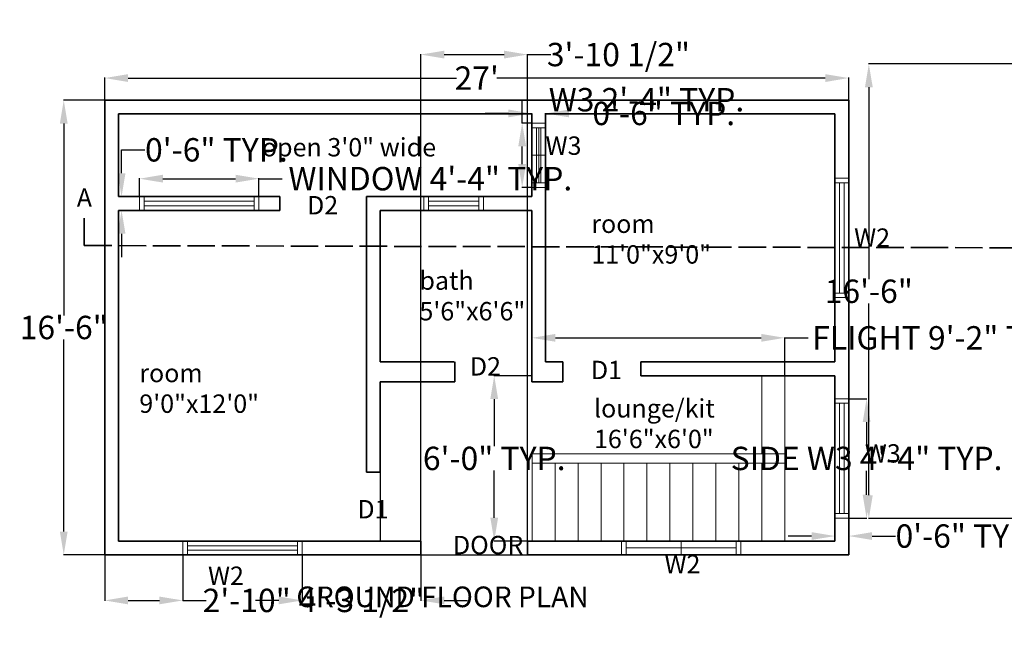
# Model space of a CAD drawing. Units: inches. Extents: x 2393 to 3270, y 740 to 1442.
# Tile 1 of 5: x 2394 to 2823, y 740 to 1008. Entities that reach past the tile are written whole.
import ezdxf

# ---------------------------------------------------------------- set-up
doc = ezdxf.new("R2010")
doc.units = ezdxf.units.IN
doc.header["$MEASUREMENT"] = 0
doc.linetypes.add('ACAD_ISO02W100', pattern=[15, 12, -3])
for name, color, linetype, lineweight in [('A-ANNO-DIMS', 2, 'Continuous', 18), ('A-ANNO-SECT', 1, 'ACAD_ISO02W100', 35), ('A-ANNO-SYMB', 3, 'Continuous', 18), ('A-ANNO-TEXT', 7, 'Continuous', 18), ('A-ANNO-TITL', 7, 'Continuous', 25), ('A-AREA-IDEN', 7, 'Continuous', 18), ('A-DOOR', 3, 'Continuous', 25), ('A-FLOR-STRS', 6, 'Continuous', 18), ('A-GLAZ', 4, 'Continuous', 18), ('A-WALL', 7, 'Continuous', 35)]:
    doc.layers.add(name, color=color, linetype=linetype, lineweight=lineweight)
doc.styles.get("Standard").update_dxf_attribs({"font": 'arial.ttf'})
doc.dimstyles.get("Standard").update_dxf_attribs({"dimtxt": 10.18, "dimasz": 10.18, "dimexe": 0.18, "dimexo": 0.0625, "dimgap": 0.09, "dimtad": 0, "dimtih": 1, "dimtoh": 1, "dimdec": 0, "dimzin": 0, "dimdsep": 46, "dimlunit": 3, "dimtxsty": 'Standard', "dimcen": 0.09, "dimadec": 0, "dimazin": 0, "dimtfac": 1, "dimtdec": 0, "dimtofl": 0, "dimtmove": 0, "dimatfit": 3, "dimfxl": 1, "dimtolj": 1, "dimtzin": 0, "dimarcsym": 0})

# ---------------------------------------------------------------- blocks, each defined once
blk = doc.blocks.new('*D1')
at = {"layer": 'A-ANNO-DIMS', "color": 0, "lineweight": -2, "transparency": 16777216}
for p, q in [((2431.27, 972.81), (2431.27, 982.53)), ((2441.45, 982.35), (2584.46, 982.35)), ((2745.09, 982.35), (2602.09, 982.35)), ((2755.27, 972.81), (2755.27, 982.53))]:
    blk.add_line(p, q, dxfattribs=at)
at = {"layer": 'A-ANNO-DIMS', "color": 0, "transparency": 16777216}
for points in [[(2441.45, 984.05), (2441.45, 980.65), (2431.27, 982.35)], [(2745.09, 984.05), (2745.09, 980.65), (2755.27, 982.35)]]:
    blk.add_solid(points, dxfattribs=at)
at = {"layer": 'Defpoints', "color": 0, "transparency": 16777216}
for p in [(2755.27, 982.35), (2431.27, 972.75), (2755.27, 972.75)]:
    blk.add_point(p, dxfattribs=at)
at = {"layer": 'A-ANNO-DIMS', "color": 0, "transparency": 16777216, "insert": (2593.27, 982.35), "char_height": 10.18, "attachment_point": 5}
blk.add_mtext("\\A1;27'", dxfattribs=at)
blk = doc.blocks.new('*D2')
at = {"layer": 'A-ANNO-DIMS', "color": 0, "lineweight": -2, "transparency": 16777216}
for p, q in [((2431.21, 972.75), (2413.26, 972.75)), ((2413.44, 962.57), (2413.44, 879.04)), ((2413.44, 784.93), (2413.44, 868.46)), ((2431.21, 774.75), (2413.26, 774.75))]:
    blk.add_line(p, q, dxfattribs=at)
at = {"layer": 'A-ANNO-DIMS', "color": 0, "transparency": 16777216}
for points in [[(2411.74, 962.57), (2415.13, 962.57), (2413.44, 972.75)], [(2411.74, 784.93), (2415.13, 784.93), (2413.44, 774.75)]]:
    blk.add_solid(points, dxfattribs=at)
at = {"layer": 'Defpoints', "color": 0, "transparency": 16777216}
for p in [(2431.27, 972.75), (2413.44, 774.75), (2431.27, 774.75)]:
    blk.add_point(p, dxfattribs=at)
at = {"layer": 'A-ANNO-DIMS', "color": 0, "transparency": 16777216, "insert": (2413.44, 873.75), "char_height": 10.18, "attachment_point": 5}
blk.add_mtext('\\A1;16\'-6"', dxfattribs=at)
blk = doc.blocks.new('WIN-52-PLAN')
for p, q in [((0, 6), (0, 0)), ((2, 6), (2, 0)), ((50, 6), (50, 0)), ((52, 6), (52, 0)), ((2, 4), (50, 4)), ((2, 2), (50, 2))]:
    blk.add_line(p, q)
blk = doc.blocks.new('WIN-26-BATH-PLAN')
for p, q in [((0, 0), (0, 6)), ((2, 0), (2, 6)), ((24, 0), (24, 6)), ((26, 0), (26, 6)), ((2, 4), (24, 4)), ((2, 2), (24, 2))]:
    blk.add_line(p, q)
blk = doc.blocks.new('WIN-W3-SIDE-PLAN')
for p, q in [((0, 52), (6, 52)), ((0, 50), (6, 50)), ((2, 50), (2, 2)), ((4, 50), (4, 2)), ((4, 50), (4, 2)), ((4, 50), (4, 2)), ((0, 2), (6, 2)), ((0, 0), (6, 0))]:
    blk.add_line(p, q)
blk = doc.blocks.new('WIN-W2-MULLION-PLAN')
for p, q in [((0, 6), (0, 0)), ((2, 6), (2, 0)), ((26, 6), (26, 0)), ((50, 6), (50, 0)), ((52, 6), (52, 0)), ((2, 3), (50, 3))]:
    blk.add_line(p, q)
blk = doc.blocks.new('WIN-W2-FRONT-PLAN')
for p, q in [((0, 6), (0, 0)), ((2, 6), (2, 0)), ((50, 6), (50, 0)), ((50, 6), (50, 0)), ((52, 6), (52, 0)), ((2, 4), (50, 4)), ((2, 2), (50, 2))]:
    blk.add_line(p, q)
blk = doc.blocks.new('WIN-W3-COURT-PLAN')
for p, q in [((0, 28), (6, 28)), ((0, 26), (6, 26)), ((2, 26), (2, 2)), ((3, 26), (3, 2)), ((4, 26), (4, 2)), ((0, 14), (6, 14)), ((0, 2), (6, 2)), ((0, 0), (6, 0))]:
    blk.add_line(p, q)
blk = doc.blocks.new('STAIR-FLIGHT-PLAN')
for p, q in [((100, 72), (100, 38)), ((100, 72), (100, 38)), ((100, 72), (100, 38)), ((110, 72), (110, 0)), ((110, 72), (110, 0)), ((110, 72), (110, 0)), ((0, 38), (0, 0)), ((110, 38), (0, 38)), ((110, 34), (0, 34)), ((10, 34), (10, 0)), ((20, 34), (20, 0)), ((30, 34), (30, 0)), ((30, 34), (30, 0)), ((30, 34), (30, 0)), ((40, 34), (40, 0)), ((50, 34), (50, 0)), ((60, 34), (60, 0)), ((70, 34), (70, 0)), ((80, 34), (80, 0)), ((80, 34), (80, 0)), ((90, 34), (90, 0)), ((100, 34), (100, 0)), ((100, 34), (100, 0)), ((100, 34), (100, 0))]:
    blk.add_line(p, q)
blk = doc.blocks.new('*D22')
at = {"layer": 'A-ANNO-DIMS', "color": 0, "lineweight": -2, "transparency": 16777216}
for p, q in [((2446.41, 930.81), (2446.41, 938.73)), ((2456.59, 938.55), (2488.23, 938.55)), ((2498.41, 930.81), (2498.41, 938.73)), ((2498.41, 938.55), (2508.59, 938.55))]:
    blk.add_line(p, q, dxfattribs=at)
at = {"layer": 'A-ANNO-DIMS', "color": 0, "transparency": 16777216}
for points in [[(2456.59, 940.25), (2456.59, 936.86), (2446.41, 938.55)], [(2488.23, 940.25), (2488.23, 936.86), (2498.41, 938.55)]]:
    blk.add_solid(points, dxfattribs=at)
at = {"layer": 'Defpoints', "color": 0, "transparency": 16777216}
for p in [(2498.41, 938.55), (2446.41, 930.75), (2498.41, 930.75)]:
    blk.add_point(p, dxfattribs=at)
at = {"layer": 'A-ANNO-DIMS', "color": 0, "transparency": 16777216, "insert": (2573.09, 938.55), "char_height": 10.18, "attachment_point": 5}
blk.add_mtext('\\A1;WINDOW 4\'-4" TYP.', dxfattribs=at)
blk = doc.blocks.new('*D23')
at = {"layer": 'A-ANNO-DIMS', "color": 0, "lineweight": -2, "transparency": 16777216}
for p, q in [((2438.61, 940.93), (2438.61, 951.11)), ((2438.61, 951.11), (2448.79, 951.11)), ((2446.35, 930.75), (2438.43, 930.75)), ((2446.35, 924.75), (2438.43, 924.75)), ((2438.61, 914.57), (2438.61, 904.39))]:
    blk.add_line(p, q, dxfattribs=at)
at = {"layer": 'A-ANNO-DIMS', "color": 0, "transparency": 16777216}
for points in [[(2436.92, 940.93), (2440.31, 940.93), (2438.61, 930.75)], [(2436.92, 914.57), (2440.31, 914.57), (2438.61, 924.75)]]:
    blk.add_solid(points, dxfattribs=at)
at = {"layer": 'Defpoints', "color": 0, "transparency": 16777216}
for p in [(2438.61, 930.75), (2446.41, 930.75), (2446.41, 924.75)]:
    blk.add_point(p, dxfattribs=at)
at = {"layer": 'A-ANNO-DIMS', "color": 0, "transparency": 16777216, "insert": (2479.91, 951.11), "char_height": 10.18, "attachment_point": 5}
blk.add_mtext('\\A1;0\'-6" TYP.', dxfattribs=at)
blk = doc.blocks.new('*D24')
at = {"layer": 'A-ANNO-DIMS', "color": 0, "lineweight": -2, "transparency": 16777216}
for p, q in [((2755.33, 842.75), (2763.25, 842.75)), ((2763.07, 832.57), (2763.07, 822.11)), ((2763.07, 800.93), (2763.07, 811.39)), ((2755.33, 790.75), (2763.25, 790.75))]:
    blk.add_line(p, q, dxfattribs=at)
at = {"layer": 'A-ANNO-DIMS', "color": 0, "transparency": 16777216}
for points in [[(2761.37, 832.57), (2764.77, 832.57), (2763.07, 842.75)], [(2761.37, 800.93), (2764.77, 800.93), (2763.07, 790.75)]]:
    blk.add_solid(points, dxfattribs=at)
at = {"layer": 'Defpoints', "color": 0, "transparency": 16777216}
for p in [(2755.27, 842.75), (2763.07, 842.75), (2755.27, 790.75)]:
    blk.add_point(p, dxfattribs=at)
at = {"layer": 'A-ANNO-DIMS', "color": 0, "transparency": 16777216, "insert": (2763.07, 816.75), "char_height": 10.18, "attachment_point": 5}
blk.add_mtext('\\A1;SIDE W3 4\'-4" TYP.', dxfattribs=at)
blk = doc.blocks.new('*D25')
at = {"layer": 'A-ANNO-DIMS', "color": 0, "lineweight": -2, "transparency": 16777216}
for p, q in [((2749.27, 790.69), (2749.27, 782.77)), ((2755.27, 790.69), (2755.27, 782.77)), ((2739.09, 782.95), (2728.91, 782.95)), ((2765.45, 782.95), (2775.63, 782.95))]:
    blk.add_line(p, q, dxfattribs=at)
at = {"layer": 'A-ANNO-DIMS', "color": 0, "transparency": 16777216}
for points in [[(2739.09, 784.65), (2739.09, 781.26), (2749.27, 782.95)], [(2765.45, 784.65), (2765.45, 781.26), (2755.27, 782.95)]]:
    blk.add_solid(points, dxfattribs=at)
at = {"layer": 'Defpoints', "color": 0, "transparency": 16777216}
for p in [(2749.27, 790.75), (2755.27, 790.75), (2755.27, 782.95)]:
    blk.add_point(p, dxfattribs=at)
at = {"layer": 'A-ANNO-DIMS', "color": 0, "transparency": 16777216, "insert": (2806.75, 782.95), "char_height": 10.18, "attachment_point": 5}
blk.add_mtext('\\A1;0\'-6" TYP.', dxfattribs=at)
blk = doc.blocks.new('*D32')
at = {"layer": 'A-ANNO-DIMS', "color": 0, "lineweight": -2, "transparency": 16777216}
for p, q in [((2613.07, 962.75), (2613.07, 972.93)), ((2613.07, 972.93), (2623.25, 972.93)), ((2617.21, 962.75), (2612.89, 962.75)), ((2613.07, 944.93), (2613.07, 952.57)), ((2617.21, 934.75), (2612.89, 934.75))]:
    blk.add_line(p, q, dxfattribs=at)
at = {"layer": 'A-ANNO-DIMS', "color": 0, "transparency": 16777216}
for points in [[(2611.37, 952.57), (2614.77, 952.57), (2613.07, 962.75)], [(2611.37, 944.93), (2614.77, 944.93), (2613.07, 934.75)]]:
    blk.add_solid(points, dxfattribs=at)
at = {"layer": 'Defpoints', "color": 0, "transparency": 16777216}
for p in [(2613.07, 962.75), (2617.27, 962.75), (2617.27, 934.75)]:
    blk.add_point(p, dxfattribs=at)
at = {"layer": 'A-ANNO-DIMS', "color": 0, "transparency": 16777216, "insert": (2667.22, 972.93), "char_height": 10.18, "attachment_point": 5}
blk.add_mtext('\\A1;W3 2\'-4" TYP.', dxfattribs=at)
blk = doc.blocks.new('*D33')
at = {"layer": 'A-ANNO-DIMS', "color": 0, "lineweight": -2, "transparency": 16777216}
for p, q in [((2607.09, 966.95), (2596.91, 966.95)), ((2617.27, 962.81), (2617.27, 967.13)), ((2623.27, 962.81), (2623.27, 967.13)), ((2633.45, 966.95), (2643.63, 966.95))]:
    blk.add_line(p, q, dxfattribs=at)
at = {"layer": 'A-ANNO-DIMS', "color": 0, "transparency": 16777216}
for points in [[(2607.09, 968.65), (2607.09, 965.26), (2617.27, 966.95)], [(2633.45, 968.65), (2633.45, 965.26), (2623.27, 966.95)]]:
    blk.add_solid(points, dxfattribs=at)
at = {"layer": 'Defpoints', "color": 0, "transparency": 16777216}
for p in [(2623.27, 966.95), (2617.27, 962.75), (2623.27, 962.75)]:
    blk.add_point(p, dxfattribs=at)
at = {"layer": 'A-ANNO-DIMS', "color": 0, "transparency": 16777216, "insert": (2674.75, 966.95), "char_height": 10.18, "attachment_point": 5}
blk.add_mtext('\\A1;0\'-6" TYP.', dxfattribs=at)
blk = doc.blocks.new('*D34')
at = {"layer": 'A-ANNO-DIMS', "color": 0, "lineweight": -2, "transparency": 16777216}
for p, q in [((2617.41, 852.81), (2617.41, 869.43)), ((2627.59, 869.25), (2717.23, 869.25)), ((2727.41, 852.81), (2727.41, 869.43)), ((2727.41, 869.25), (2737.59, 869.25))]:
    blk.add_line(p, q, dxfattribs=at)
at = {"layer": 'A-ANNO-DIMS', "color": 0, "transparency": 16777216}
for points in [[(2627.59, 870.95), (2627.59, 867.56), (2617.41, 869.25)], [(2717.23, 870.95), (2717.23, 867.56), (2727.41, 869.25)]]:
    blk.add_solid(points, dxfattribs=at)
at = {"layer": 'Defpoints', "color": 0, "transparency": 16777216}
for p in [(2727.41, 869.25), (2617.41, 852.75), (2727.41, 852.75)]:
    blk.add_point(p, dxfattribs=at)
at = {"layer": 'A-ANNO-DIMS', "color": 0, "transparency": 16777216, "insert": (2795.67, 869.25), "char_height": 10.18, "attachment_point": 5}
blk.add_mtext('\\A1;FLIGHT 9\'-2" TYP.', dxfattribs=at)
blk = doc.blocks.new('*D35')
at = {"layer": 'A-ANNO-DIMS', "color": 0, "lineweight": -2, "transparency": 16777216}
for p, q in [((2617.34, 852.75), (2600.73, 852.75)), ((2600.91, 842.57), (2600.91, 822.04)), ((2600.91, 790.93), (2600.91, 811.46)), ((2617.34, 780.75), (2600.73, 780.75))]:
    blk.add_line(p, q, dxfattribs=at)
at = {"layer": 'A-ANNO-DIMS', "color": 0, "transparency": 16777216}
for points in [[(2599.21, 842.57), (2602.6, 842.57), (2600.91, 852.75)], [(2599.21, 790.93), (2602.6, 790.93), (2600.91, 780.75)]]:
    blk.add_solid(points, dxfattribs=at)
at = {"layer": 'Defpoints', "color": 0, "transparency": 16777216}
for p in [(2600.91, 852.75), (2617.41, 852.75), (2617.41, 780.75)]:
    blk.add_point(p, dxfattribs=at)
at = {"layer": 'A-ANNO-DIMS', "color": 0, "transparency": 16777216, "insert": (2600.91, 816.75), "char_height": 10.18, "attachment_point": 5}
blk.add_mtext('\\A1;6\'-0" TYP.', dxfattribs=at)
blk = doc.blocks.new('*D46')
at = {"layer": 'A-ANNO-DIMS', "color": 0, "lineweight": -2, "transparency": 16777216}
for p, q in [((2431.27, 774.69), (2431.27, 754.74)), ((2465.27, 774.69), (2465.27, 754.74)), ((2441.45, 754.92), (2455.09, 754.92)), ((2465.27, 754.92), (2475.45, 754.92))]:
    blk.add_line(p, q, dxfattribs=at)
at = {"layer": 'A-ANNO-DIMS', "color": 0, "transparency": 16777216}
for points in [[(2441.45, 756.61), (2441.45, 753.22), (2431.27, 754.92)], [(2455.09, 756.61), (2455.09, 753.22), (2465.27, 754.92)]]:
    blk.add_solid(points, dxfattribs=at)
at = {"layer": 'Defpoints', "color": 0, "transparency": 16777216}
for p in [(2431.27, 774.75), (2465.27, 774.75), (2465.27, 754.92)]:
    blk.add_point(p, dxfattribs=at)
at = {"layer": 'A-ANNO-DIMS', "color": 0, "transparency": 16777216, "insert": (2493.11, 754.92), "char_height": 10.18, "attachment_point": 5}
blk.add_mtext('\\A1;2\'-10"', dxfattribs=at)
blk = doc.blocks.new('*D47')
at = {"layer": 'A-ANNO-DIMS', "color": 0, "lineweight": -2, "transparency": 16777216}
for p, q in [((2517.27, 774.69), (2517.27, 754.74)), ((2568.93, 774.69), (2568.93, 754.74)), ((2507.09, 754.92), (2496.91, 754.92)), ((2579.11, 754.92), (2589.29, 754.92))]:
    blk.add_line(p, q, dxfattribs=at)
at = {"layer": 'A-ANNO-DIMS', "color": 0, "transparency": 16777216}
for points in [[(2507.09, 756.61), (2507.09, 753.22), (2517.27, 754.92)], [(2579.11, 756.61), (2579.11, 753.22), (2568.93, 754.92)]]:
    blk.add_solid(points, dxfattribs=at)
at = {"layer": 'Defpoints', "color": 0, "transparency": 16777216}
for p in [(2517.27, 774.75), (2568.93, 774.75), (2568.93, 754.92)]:
    blk.add_point(p, dxfattribs=at)
at = {"layer": 'A-ANNO-DIMS', "color": 0, "transparency": 16777216, "insert": (2543.1, 754.92), "char_height": 10.18, "attachment_point": 5}
blk.add_mtext('\\A1;4\'-3 1/2"', dxfattribs=at)
blk = doc.blocks.new('*D48')
at = {"layer": 'A-ANNO-DIMS', "color": 0, "lineweight": -2, "transparency": 16777216}
for p, q in [((2568.93, 780.81), (2568.93, 992.77)), ((2579.11, 992.59), (2605.22, 992.59)), ((2615.4, 780.81), (2615.4, 992.77)), ((2615.4, 992.59), (2625.58, 992.59))]:
    blk.add_line(p, q, dxfattribs=at)
at = {"layer": 'A-ANNO-DIMS', "color": 0, "transparency": 16777216}
for points in [[(2579.11, 994.28), (2579.11, 990.89), (2568.93, 992.59)], [(2605.22, 994.28), (2605.22, 990.89), (2615.4, 992.59)]]:
    blk.add_solid(points, dxfattribs=at)
at = {"layer": 'Defpoints', "color": 0, "transparency": 16777216}
for p in [(2615.4, 992.59), (2568.93, 780.75), (2615.4, 780.75)]:
    blk.add_point(p, dxfattribs=at)
at = {"layer": 'A-ANNO-DIMS', "color": 0, "transparency": 16777216, "insert": (2655.01, 992.59), "char_height": 10.18, "attachment_point": 5}
blk.add_mtext('\\A1;3\'-10 1/2"', dxfattribs=at)
blk = doc.blocks.new('*D54')
at = {"layer": 'A-ANNO-DIMS', "color": 0, "lineweight": -2, "transparency": 16777216}
for p, q in [((2873.72, 988.53), (2763.87, 988.53)), ((2764.05, 978.35), (2764.05, 894.82)), ((2764.05, 800.71), (2764.05, 884.25)), ((2873.72, 790.53), (2763.87, 790.53))]:
    blk.add_line(p, q, dxfattribs=at)
at = {"layer": 'A-ANNO-DIMS', "color": 0, "transparency": 16777216}
for points in [[(2762.35, 978.35), (2765.75, 978.35), (2764.05, 988.53)], [(2762.35, 800.71), (2765.75, 800.71), (2764.05, 790.53)]]:
    blk.add_solid(points, dxfattribs=at)
at = {"layer": 'Defpoints', "color": 0, "transparency": 16777216}
for p in [(2764.05, 988.53), (2873.78, 988.53), (2873.78, 790.53)]:
    blk.add_point(p, dxfattribs=at)
at = {"layer": 'A-ANNO-DIMS', "color": 0, "transparency": 16777216, "insert": (2764.05, 889.53), "char_height": 10.18, "attachment_point": 5}
blk.add_mtext('\\A1;16\'-6"', dxfattribs=at)

msp = doc.modelspace()

# ---------------------------------------------------------------- linework, layer by layer
at = {"layer": 'A-ANNO-SECT'}
for p, q in [((2422.3, 909.42), (2422.33, 923.42)), ((2422.3, 909.42), (2786.62, 908.53)), ((2786.62, 908.53), (3228.37, 908.02))]:
    msp.add_line(p, q, dxfattribs=at)
at = {"layer": 'A-DOOR'}
for p, q in [((2551.27, 810.75), (2551.27, 780.75)), ((2568.93, 774.75), (2615.4, 774.75))]:
    msp.add_line(p, q, dxfattribs=at)
at = {"layer": 'A-WALL'}
for p, q in [((2431.27, 774.75), (2431.27, 972.75)), ((2431.27, 972.75), (2755.27, 972.75)), ((2755.27, 972.75), (2755.27, 774.75)), ((2437.27, 966.75), (2545.27, 966.75)), ((2437.27, 930.75), (2437.27, 966.75)), ((2545.27, 966.75), (2551.27, 966.75)), ((2551.27, 966.75), (2617.27, 966.75)), ((2617.27, 930.75), (2617.27, 966.75)), ((2623.27, 858.75), (2623.27, 966.75)), ((2623.27, 966.75), (2749.27, 966.75)), ((2749.27, 966.75), (2749.27, 858.75)), ((2507.55, 930.75), (2437.27, 930.75)), ((2507.55, 930.75), (2507.55, 924.75)), ((2545.27, 930.75), (2545.27, 924.75)), ((2551.27, 930.75), (2545.27, 930.75)), ((2617.27, 930.75), (2551.27, 930.75)), ((2507.55, 924.75), (2437.27, 924.75)), ((2437.27, 846.75), (2437.27, 924.75)), ((2545.27, 846.75), (2545.27, 924.75)), ((2617.27, 924.75), (2551.27, 924.75)), ((2551.27, 858.75), (2551.27, 924.75)), ((2617.27, 924.75), (2617.27, 850.11)), ((2551.27, 858.75), (2583.44, 858.75)), ((2583.72, 850.11), (2583.72, 858.75)), ((2623.27, 858.75), (2630.84, 858.75)), ((2630.84, 858.75), (2630.84, 852.75)), ((2664.8, 858.75), (2664.8, 852.75)), ((2664.8, 858.75), (2749.27, 858.75)), ((2551.27, 846.75), (2551.27, 850.11)), ((2551.27, 850.11), (2583.72, 850.11)), ((2617.27, 850.11), (2623.27, 850.11)), ((2623.27, 850.11), (2630.84, 850.11)), ((2630.84, 850.11), (2630.84, 852.75)), ((2664.8, 852.75), (2749.27, 852.75)), ((2749.27, 852.75), (2749.27, 780.75)), ((2437.27, 840.75), (2437.27, 846.75)), ((2545.27, 840.75), (2545.27, 846.75)), ((2551.27, 846.75), (2551.27, 840.75)), ((2437.27, 780.75), (2437.27, 840.75)), ((2545.27, 810.75), (2545.27, 840.75)), ((2551.27, 810.75), (2551.27, 840.75)), ((2545.27, 810.75), (2551.27, 810.75)), ((2545.27, 780.75), (2437.27, 780.75)), ((2545.27, 780.75), (2551.27, 780.75)), ((2568.93, 780.75), (2551.27, 780.75)), ((2568.93, 780.75), (2568.93, 774.75)), ((2749.27, 780.75), (2615.4, 780.75)), ((2615.4, 780.75), (2615.4, 774.75)), ((2568.93, 774.75), (2431.27, 774.75)), ((2755.27, 774.75), (2615.4, 774.75))]:
    msp.add_line(p, q, dxfattribs=at)

# ---------------------------------------------------------------- block references
at = {"layer": 'A-FLOR-STRS'}
msp.add_blockref('STAIR-FLIGHT-PLAN', (2617.41, 780.75), dxfattribs=at)
at = {"layer": 'A-GLAZ'}
for name, p in [('WIN-W3-COURT-PLAN', (2617.27, 934.75)), ('WIN-52-PLAN', (2446.41, 924.75)), ('WIN-26-BATH-PLAN', (2570.27, 924.75)), ('WIN-W3-SIDE-PLAN', (2749.27, 790.75)), ('WIN-W2-FRONT-PLAN', (2465.27, 774.75)), ('WIN-W2-MULLION-PLAN', (2656.34, 774.75))]:
    msp.add_blockref(name, p, dxfattribs=at)
at = {"layer": 'A-GLAZ', "rotation": 89.99999999999721}
msp.add_blockref('WIN-52-PLAN', (2755.27, 886.75), dxfattribs=at)

# ---------------------------------------------------------------- texts
at = {"layer": 'A-ANNO-SYMB', "insert": (2419.11, 934.3), "char_height": 8, "attachment_point": 1}
msp.add_mtext_dynamic_manual_height_columns('A', width=76.737, gutter_width=1, heights=[0], dxfattribs=at)
at = {"layer": 'A-ANNO-TEXT', "char_height": 8, "attachment_point": 1}
for s, insert in [('W3', (2623.27, 956.93)), ('D2', (2519.38, 930.99)), ('W2', (2757.66, 916.88)), ('D2', (2590.29, 860.83)), ('D1', (2643, 859.26)), ('W3', (2762.31, 822.93)), ('D1', (2541.3, 798.63)), ('DOOR', (2582.91, 783.03)), ('W2', (2675.07, 774.74)), ('W2', (2476.26, 769.68))]:
    msp.add_mtext_dynamic_manual_height_columns(s, width=76.737, gutter_width=1, heights=[0], dxfattribs=dict(at, insert=insert))
at = {"layer": 'A-ANNO-TITL', "insert": (2514.75, 760.98), "char_height": 9, "attachment_point": 1}
msp.add_mtext_dynamic_manual_height_columns('GROUND FLOOR PLAN', width=140.3126, gutter_width=1, heights=[0], dxfattribs=at)
at = {"layer": 'A-AREA-IDEN', "char_height": 8, "attachment_point": 1}
for s, insert in [('open 3\'0" wide', (2499.72, 956.23)), ('room\\P11\'0"x9\'0"', (2643.19, 922.91)), ('bath\\P5\'6"x6\'6"', (2568.34, 898.18)), ('room\\P9\'0"x12\'0"', (2446.34, 857.93)), ('lounge/kit\\P16\'6"x6\'0"', (2644.35, 842.56))]:
    msp.add_mtext_dynamic_manual_height_columns(s, width=76.737, gutter_width=1, heights=[0], dxfattribs=dict(at, insert=insert))

# ---------------------------------------------------------------- dimensions: what is measured, and where the dimension line sits
at = {"layer": 'A-ANNO-DIMS'}
for base, p1, p2, override, picture, middle in [((2615.4, 992.59), (2568.93, 780.75), (2615.4, 780.75), {"dimdec": 1, "dimlfac": 1, "dimrnd": 0, "dimzin": 1, "dimdsep": 46, "dimlunit": 4, "dimfrac": 2}, '*D48', (2655.01, 992.59)), ((2755.27, 982.35), (2431.27, 972.75), (2755.27, 972.75), {"dimclrd": 0, "dimclre": 0, "dimclrt": 0}, '*D1', (2593.27, 982.35)), ((2465.27, 754.92), (2431.27, 774.75), (2465.27, 774.75), {"dimdec": 1, "dimlfac": 1, "dimrnd": 0, "dimzin": 1, "dimdsep": 46, "dimlunit": 4, "dimfrac": 2}, '*D46', (2493.11, 754.92)), ((2568.93, 754.92), (2517.27, 774.75), (2568.93, 774.75), {"dimdec": 1, "dimlfac": 1, "dimrnd": 0, "dimzin": 1, "dimdsep": 46, "dimlunit": 4, "dimfrac": 2}, '*D47', (2543.1, 754.92))]:
    dim = msp.add_linear_dim(base=base, p1=p1, p2=p2, dimstyle='Standard', override=override, dxfattribs=at)
    dim.commit()
    dim.dimension.update_dxf_attribs({"geometry": picture, "text_midpoint": middle})
for base, p1, p2, text, picture, middle in [((2613.07, 962.75), (2617.27, 934.75), (2617.27, 962.75), 'W3 <> TYP.', '*D32', (2667.22, 972.93)), ((2438.61, 930.75), (2446.41, 924.75), (2446.41, 930.75), '<> TYP.', '*D23', (2479.91, 951.11)), ((2600.91, 852.75), (2617.41, 780.75), (2617.41, 852.75), '<> TYP.', '*D35', (2600.91, 816.75)), ((2763.07, 842.75), (2755.27, 790.75), (2755.27, 842.75), 'SIDE W3 <> TYP.', '*D24', (2763.07, 816.75))]:
    dim = msp.add_linear_dim(base=base, p1=p1, p2=p2, angle=90, text=text, dimstyle='Standard', override={"dimdec": 1, "dimlfac": 1, "dimrnd": 0, "dimzin": 1, "dimdsep": 46, "dimlunit": 4, "dimfrac": 2}, dxfattribs=at)
    dim.commit()
    dim.dimension.update_dxf_attribs({"geometry": picture, "text_midpoint": middle})
for base, p1, p2, override, picture, middle in [((2764.05, 988.53), (2873.78, 790.53), (2873.78, 988.53), {"dimdec": 1, "dimlfac": 1, "dimrnd": 0, "dimzin": 1, "dimdsep": 46, "dimlunit": 4, "dimfrac": 2}, '*D54', (2764.05, 889.53)), ((2413.44, 774.75), (2431.27, 972.75), (2431.27, 774.75), {"dimclrd": 0, "dimclre": 0, "dimclrt": 0}, '*D2', (2413.44, 873.75))]:
    dim = msp.add_linear_dim(base=base, p1=p1, p2=p2, angle=90, dimstyle='Standard', override=override, dxfattribs=at)
    dim.commit()
    dim.dimension.update_dxf_attribs({"geometry": picture, "text_midpoint": middle})
for base, p1, p2, text, picture, middle in [((2623.27, 966.95), (2617.27, 962.75), (2623.27, 962.75), '<> TYP.', '*D33', (2674.75, 966.95)), ((2498.41, 938.55), (2446.41, 930.75), (2498.41, 930.75), 'WINDOW <> TYP.', '*D22', (2573.09, 938.55)), ((2727.41, 869.25), (2617.41, 852.75), (2727.41, 852.75), 'FLIGHT <> TYP.', '*D34', (2795.67, 869.25)), ((2755.27, 782.95), (2749.27, 790.75), (2755.27, 790.75), '<> TYP.', '*D25', (2806.75, 782.95))]:
    dim = msp.add_linear_dim(base=base, p1=p1, p2=p2, text=text, dimstyle='Standard', override={"dimdec": 1, "dimlfac": 1, "dimrnd": 0, "dimzin": 1, "dimdsep": 46, "dimlunit": 4, "dimfrac": 2}, dxfattribs=at)
    dim.commit()
    dim.dimension.update_dxf_attribs({"geometry": picture, "text_midpoint": middle})

doc.saveas('drawing.dxf')
